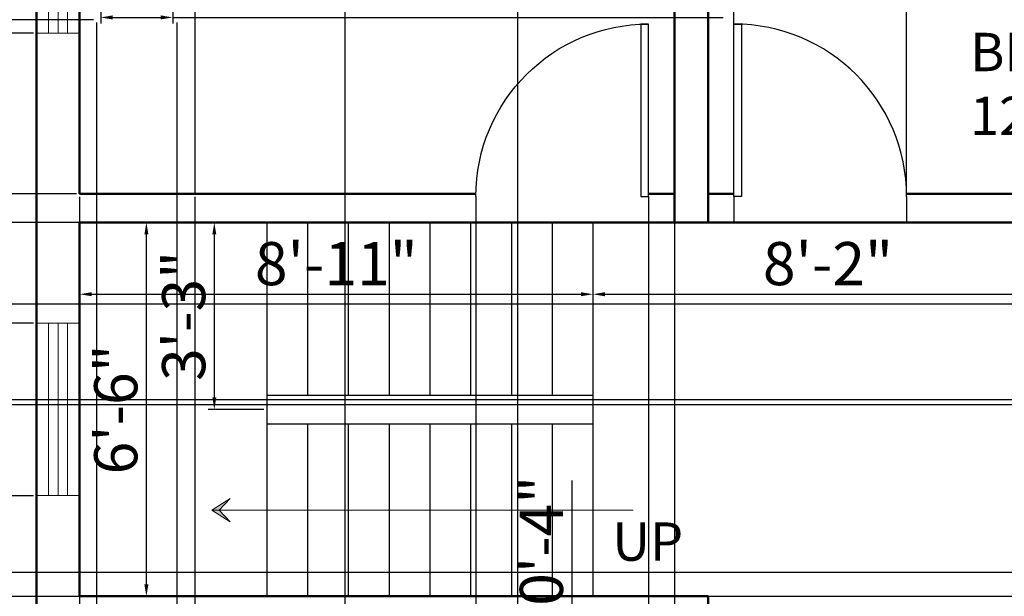
# Model space of a CAD drawing. Units: inches. Extents: x 2181 to 2717, y 1819 to 2296.
# Tile 3 of 5: x 2326 to 2531, y 2036 to 2157. Entities that reach past the tile are written whole.
import ezdxf

# ---------------------------------------------------------------- set-up
doc = ezdxf.new("R2010")
doc.units = ezdxf.units.IN
for name, color, linetype, lineweight in [('A-ANNO-DIMS', 2, 'Continuous', 13), ('A-ANNO-SYMB', 7, 'Continuous', 18), ('A-ANNO-SYMB-PATT', 7, 'Continuous', 18), ('A-ANNO-TEXT', 7, 'Continuous', 18), ('A-AREA-IDEN', 7, 'Continuous', 25), ('A-DOOR', 3, 'Continuous', 25), ('A-FLOR-CASE', 32, 'Continuous', 25), ('A-FLOR-STRS', 7, 'Continuous', 25), ('A-GLAZ', 4, 'Continuous', 18), ('A-WALL', 7, 'Continuous', 50)]:
    doc.layers.add(name, color=color, linetype=linetype, lineweight=lineweight)
doc.styles.get("Standard").update_dxf_attribs({"font": 'arial.ttf'})
doc.dimstyles.new('ISO-25', dxfattribs={"dimtxt": 9, "dimasz": 2.5, "dimexe": 1.25, "dimexo": 0.625, "dimtad": 1, "dimlunit": 3, "dimtxsty": 'Standard', "dimcen": 2.5, "dimadec": 0, "dimazin": 0, "dimtfac": 1, "dimtmove": 0, "dimatfit": 3, "dimfxl": 1, "dimarcsym": 0})

# ---------------------------------------------------------------- blocks, each defined once
blk = doc.blocks.new('*U2')
for p, q in [((0, 0), (0, -6)), ((40, 0), (40, -6))]:
    blk.add_line(p, q)
blk.add_lwpolyline([(0, 0), (0, 40), (1.75, 40), (1.75, 0)], close=True)
blk.add_arc((0, 0), 40, 0, 90)
blk = doc.blocks.new('*D10')
at = {"layer": 'A-ANNO-DIMS', "color": 0, "lineweight": -2, "transparency": 16777216}
for p, q in [((2338.97, 2114.2), (2353.51, 2114.2)), ((2352.26, 2038.7), (2352.26, 2111.7)), ((2338.97, 2036.2), (2353.51, 2036.2))]:
    blk.add_line(p, q, dxfattribs=at)
at = {"layer": 'A-ANNO-DIMS', "color": 0, "transparency": 16777216}
for points in [[(2351.84, 2111.7), (2352.68, 2111.7), (2352.26, 2114.2)], [(2351.84, 2038.7), (2352.68, 2038.7), (2352.26, 2036.2)]]:
    blk.add_solid(points, dxfattribs=at)
at = {"layer": 'Defpoints', "color": 0, "transparency": 16777216}
for p in [(2338.35, 2114.2), (2352.26, 2114.2), (2338.35, 2036.2)]:
    blk.add_point(p, dxfattribs=at)
at = {"layer": 'A-ANNO-DIMS', "color": 0, "transparency": 16777216, "insert": (2347.04, 2075.2), "char_height": 9, "attachment_point": 5, "rotation": 90}
blk.add_mtext('6\'-6"', dxfattribs=at)
blk = doc.blocks.new('*D11')
at = {"layer": 'A-ANNO-DIMS', "color": 0, "lineweight": -2, "transparency": 16777216}
for p, q in [((2376.72, 2114.2), (2365.17, 2114.2)), ((2366.42, 2111.7), (2366.42, 2077.7)), ((2376.72, 2075.2), (2365.17, 2075.2))]:
    blk.add_line(p, q, dxfattribs=at)
at = {"layer": 'A-ANNO-DIMS', "color": 0, "transparency": 16777216}
for points in [[(2366.01, 2111.7), (2366.84, 2111.7), (2366.42, 2114.2)], [(2366.01, 2077.7), (2366.84, 2077.7), (2366.42, 2075.2)]]:
    blk.add_solid(points, dxfattribs=at)
at = {"layer": 'Defpoints', "color": 0, "transparency": 16777216}
for p in [(2377.35, 2114.2), (2366.42, 2075.2), (2377.35, 2075.2)]:
    blk.add_point(p, dxfattribs=at)
at = {"layer": 'A-ANNO-DIMS', "color": 0, "transparency": 16777216, "insert": (2361.2, 2094.7), "char_height": 9, "attachment_point": 5, "rotation": 90}
blk.add_mtext('3\'-3"', dxfattribs=at)
blk = doc.blocks.new('*D12')
at = {"layer": 'A-ANNO-DIMS', "color": 0, "lineweight": -2, "transparency": 16777216}
for p, q in [((2338.35, 2113.58), (2338.35, 2097.98)), ((2445.35, 2113.58), (2445.35, 2097.98)), ((2340.85, 2099.23), (2442.85, 2099.23))]:
    blk.add_line(p, q, dxfattribs=at)
at = {"layer": 'A-ANNO-DIMS', "color": 0, "transparency": 16777216}
for points in [[(2340.85, 2099.65), (2340.85, 2098.81), (2338.35, 2099.23)], [(2442.85, 2099.65), (2442.85, 2098.81), (2445.35, 2099.23)]]:
    blk.add_solid(points, dxfattribs=at)
at = {"layer": 'Defpoints', "color": 0, "transparency": 16777216}
for p in [(2338.35, 2114.2), (2445.35, 2114.2), (2445.35, 2099.23)]:
    blk.add_point(p, dxfattribs=at)
at = {"layer": 'A-ANNO-DIMS', "color": 0, "transparency": 16777216, "insert": (2391.85, 2104.45), "char_height": 9, "attachment_point": 5}
blk.add_mtext('8\'-11"', dxfattribs=at)
blk = doc.blocks.new('*D13')
at = {"layer": 'A-ANNO-DIMS', "color": 0, "lineweight": -2, "transparency": 16777216}
for p, q in [((2445.35, 2113.58), (2445.35, 2097.98)), ((2543.35, 2113.58), (2543.35, 2097.98)), ((2447.85, 2099.23), (2540.85, 2099.23))]:
    blk.add_line(p, q, dxfattribs=at)
at = {"layer": 'A-ANNO-DIMS', "color": 0, "transparency": 16777216}
for points in [[(2447.85, 2099.65), (2447.85, 2098.81), (2445.35, 2099.23)], [(2540.85, 2099.65), (2540.85, 2098.81), (2543.35, 2099.23)]]:
    blk.add_solid(points, dxfattribs=at)
at = {"layer": 'Defpoints', "color": 0, "transparency": 16777216}
for p in [(2445.35, 2114.2), (2543.35, 2114.2), (2543.35, 2099.23)]:
    blk.add_point(p, dxfattribs=at)
at = {"layer": 'A-ANNO-DIMS', "color": 0, "transparency": 16777216, "insert": (2494.35, 2104.45), "char_height": 9, "attachment_point": 5}
blk.add_mtext('8\'-2"', dxfattribs=at)
blk = doc.blocks.new('WIN-60IN')
for p, q in [((0, 0), (0, 9)), ((60, 0), (60, 9)), ((60, 6.5), (0, 6.5)), ((60, 4.5), (0, 4.5)), ((60, 2.5), (0, 2.5))]:
    blk.add_line(p, q)
blk = doc.blocks.new('*D19')
at = {"layer": 'A-ANNO-DIMS', "color": 0, "lineweight": -2, "transparency": 16777216}
for p, q in [((2338.35, 1997.93), (2181.23, 1997.93)), ((2338.35, 1986.33), (2338.35, 1999.18)), ((2417.32, 1997.93), (2340.85, 1997.93)), ((2419.82, 1986.33), (2419.82, 1999.18))]:
    blk.add_line(p, q, dxfattribs=at)
at = {"layer": 'A-ANNO-DIMS', "color": 0, "transparency": 16777216}
for points in [[(2340.85, 1998.34), (2340.85, 1997.51), (2338.35, 1997.93)], [(2417.32, 1998.34), (2417.32, 1997.51), (2419.82, 1997.93)]]:
    blk.add_solid(points, dxfattribs=at)
at = {"layer": 'Defpoints', "color": 0, "transparency": 16777216}
for p in [(2338.35, 1997.93), (2338.35, 1985.7), (2419.82, 1985.7)]:
    blk.add_point(p, dxfattribs=at)
at = {"layer": 'A-ANNO-DIMS', "color": 0, "transparency": 16777216, "insert": (2258.54, 2003.48), "char_height": 9, "attachment_point": 5}
blk.add_mtext('QUEEN BED 6\'-9 1/2" TYP.', dxfattribs=at)
blk = doc.blocks.new('*D21')
at = {"layer": 'A-ANNO-DIMS', "color": 0, "lineweight": -2, "transparency": 16777216}
for p, q in [((2342.73, 2158.61), (2342.73, 2155.73)), ((2357.74, 2158.61), (2357.74, 2155.73)), ((2345.23, 2156.98), (2355.24, 2156.98)), ((2357.74, 2156.98), (2472.54, 2156.98))]:
    blk.add_line(p, q, dxfattribs=at)
at = {"layer": 'A-ANNO-DIMS', "color": 0, "transparency": 16777216}
for points in [[(2345.23, 2157.4), (2345.23, 2156.56), (2342.73, 2156.98)], [(2355.24, 2157.4), (2355.24, 2156.56), (2357.74, 2156.98)]]:
    blk.add_solid(points, dxfattribs=at)
at = {"layer": 'Defpoints', "color": 0, "transparency": 16777216}
for p in [(2342.73, 2159.23), (2357.74, 2159.23), (2357.74, 2156.98)]:
    blk.add_point(p, dxfattribs=at)
at = {"layer": 'A-ANNO-DIMS', "color": 0, "transparency": 16777216, "insert": (2416.39, 2162.2), "char_height": 9, "attachment_point": 5}
blk.add_mtext('BURNER 1\'-3" TYP.', dxfattribs=at)
blk = doc.blocks.new('*D27')
at = {"layer": 'A-ANNO-DIMS', "color": 0, "lineweight": -2, "transparency": 16777216}
for p, q in [((2328.72, 2093.2), (2306.75, 2093.2)), ((2308, 2090.7), (2308, 2059.7)), ((2328.72, 2057.2), (2306.75, 2057.2))]:
    blk.add_line(p, q, dxfattribs=at)
at = {"layer": 'A-ANNO-DIMS', "color": 0, "transparency": 16777216}
for points in [[(2307.58, 2090.7), (2308.41, 2090.7), (2308, 2093.2)], [(2307.58, 2059.7), (2308.41, 2059.7), (2308, 2057.2)]]:
    blk.add_solid(points, dxfattribs=at)
at = {"layer": 'Defpoints', "color": 0, "transparency": 16777216}
for p in [(2329.35, 2093.2), (2308, 2057.2), (2329.35, 2057.2)]:
    blk.add_point(p, dxfattribs=at)
at = {"layer": 'A-ANNO-DIMS', "color": 0, "transparency": 16777216, "insert": (2302.77, 2075.2), "char_height": 9, "attachment_point": 5, "rotation": 90}
blk.add_mtext('3\'-0"', dxfattribs=at)
blk = doc.blocks.new('*D28')
at = {"layer": 'A-ANNO-DIMS', "color": 0, "lineweight": -2, "transparency": 16777216}
for p, q in [((2328.72, 2153.7), (2306.75, 2153.7)), ((2308, 2095.7), (2308, 2151.2)), ((2328.72, 2093.2), (2306.75, 2093.2))]:
    blk.add_line(p, q, dxfattribs=at)
at = {"layer": 'A-ANNO-DIMS', "color": 0, "transparency": 16777216}
for points in [[(2307.58, 2151.2), (2308.41, 2151.2), (2308, 2153.7)], [(2307.58, 2095.7), (2308.41, 2095.7), (2308, 2093.2)]]:
    blk.add_solid(points, dxfattribs=at)
at = {"layer": 'Defpoints', "color": 0, "transparency": 16777216}
for p in [(2308, 2153.7), (2329.35, 2153.7), (2329.35, 2093.2)]:
    blk.add_point(p, dxfattribs=at)
at = {"layer": 'A-ANNO-DIMS', "color": 0, "transparency": 16777216, "insert": (2302.72, 2123.45), "char_height": 9, "attachment_point": 5, "rotation": 90}
blk.add_mtext('5\'-0 1/2"', dxfattribs=at)
blk = doc.blocks.new('*D40')
at = {"layer": 'A-ANNO-DIMS', "color": 0, "lineweight": -2, "transparency": 16777216}
for p, q in [((2474.75, 2120.83), (2474.75, 2278.8)), ((2510.75, 2120.83), (2510.75, 2278.8)), ((2477.25, 2277.55), (2508.25, 2277.55))]:
    blk.add_line(p, q, dxfattribs=at)
at = {"layer": 'A-ANNO-DIMS', "color": 0, "transparency": 16777216}
for points in [[(2477.25, 2277.97), (2477.25, 2277.14), (2474.75, 2277.55)], [(2508.25, 2277.97), (2508.25, 2277.14), (2510.75, 2277.55)]]:
    blk.add_solid(points, dxfattribs=at)
at = {"layer": 'Defpoints', "color": 0, "transparency": 16777216}
for p in [(2510.75, 2277.55), (2474.75, 2120.2), (2510.75, 2120.2)]:
    blk.add_point(p, dxfattribs=at)
at = {"layer": 'A-ANNO-DIMS', "color": 0, "transparency": 16777216, "insert": (2492.75, 2282.78), "char_height": 9, "attachment_point": 5}
blk.add_mtext('3\'-0"', dxfattribs=at)
blk = doc.blocks.new('*D41')
at = {"layer": 'A-ANNO-DIMS', "color": 0, "lineweight": -2, "transparency": 16777216}
for p, q in [((2338.35, 2119.58), (2338.35, 1825.6)), ((2362.35, 2119.58), (2362.35, 1825.6)), ((2340.85, 1826.85), (2359.85, 1826.85)), ((2362.35, 1826.85), (2390.17, 1826.85))]:
    blk.add_line(p, q, dxfattribs=at)
at = {"layer": 'A-ANNO-DIMS', "color": 0, "transparency": 16777216}
for points in [[(2340.85, 1827.27), (2340.85, 1826.44), (2338.35, 1826.85)], [(2359.85, 1827.27), (2359.85, 1826.44), (2362.35, 1826.85)]]:
    blk.add_solid(points, dxfattribs=at)
at = {"layer": 'Defpoints', "color": 0, "transparency": 16777216}
for p in [(2338.35, 2120.2), (2362.35, 2120.2), (2362.35, 1826.85)]:
    blk.add_point(p, dxfattribs=at)
at = {"layer": 'A-ANNO-DIMS', "color": 0, "transparency": 16777216, "insert": (2377.51, 1832.07), "char_height": 9, "attachment_point": 5}
blk.add_mtext('2\'-0"', dxfattribs=at)
blk = doc.blocks.new('*D43')
at = {"layer": 'A-ANNO-DIMS', "color": 0, "lineweight": -2, "transparency": 16777216}
for p, q in [((2393.61, 2225.64), (2393.61, 1825.6)), ((2429.61, 2225.64), (2429.61, 1825.6)), ((2396.11, 1826.85), (2427.11, 1826.85))]:
    blk.add_line(p, q, dxfattribs=at)
at = {"layer": 'A-ANNO-DIMS', "color": 0, "transparency": 16777216}
for points in [[(2396.11, 1827.27), (2396.11, 1826.44), (2393.61, 1826.85)], [(2427.11, 1827.27), (2427.11, 1826.44), (2429.61, 1826.85)]]:
    blk.add_solid(points, dxfattribs=at)
at = {"layer": 'Defpoints', "color": 0, "transparency": 16777216}
for p in [(2393.61, 2226.26), (2429.61, 2226.26), (2429.61, 1826.85)]:
    blk.add_point(p, dxfattribs=at)
at = {"layer": 'A-ANNO-DIMS', "color": 0, "transparency": 16777216, "insert": (2411.61, 1832.08), "char_height": 9, "attachment_point": 5}
blk.add_mtext('3\'-0"', dxfattribs=at)
blk = doc.blocks.new('*D45')
at = {"layer": 'A-ANNO-DIMS', "color": 0, "lineweight": -2, "transparency": 16777216}
for p, q in [((2429.61, 2225.64), (2429.61, 1825.6)), ((2462.35, 2222.58), (2462.35, 1825.6)), ((2432.11, 1826.85), (2459.85, 1826.85)), ((2462.35, 1826.85), (2511.15, 1826.85))]:
    blk.add_line(p, q, dxfattribs=at)
at = {"layer": 'A-ANNO-DIMS', "color": 0, "transparency": 16777216}
for points in [[(2432.11, 1827.27), (2432.11, 1826.44), (2429.61, 1826.85)], [(2459.85, 1827.27), (2459.85, 1826.44), (2462.35, 1826.85)]]:
    blk.add_solid(points, dxfattribs=at)
at = {"layer": 'Defpoints', "color": 0, "transparency": 16777216}
for p in [(2429.61, 2226.26), (2462.35, 2223.2), (2462.35, 1826.85)]:
    blk.add_point(p, dxfattribs=at)
at = {"layer": 'A-ANNO-DIMS', "color": 0, "transparency": 16777216, "insert": (2488, 1832.13), "char_height": 9, "attachment_point": 5}
blk.add_mtext('2\'-8 1/2"', dxfattribs=at)
blk = doc.blocks.new('*D46')
at = {"layer": 'A-ANNO-DIMS', "color": 0, "lineweight": -2, "transparency": 16777216}
for p, q in [((2341.24, 2198.7), (2306.75, 2198.7)), ((2308, 2159.01), (2308, 2196.2)), ((2341.24, 2156.51), (2306.75, 2156.51))]:
    blk.add_line(p, q, dxfattribs=at)
at = {"layer": 'A-ANNO-DIMS', "color": 0, "transparency": 16777216}
for points in [[(2307.58, 2196.2), (2308.41, 2196.2), (2308, 2198.7)], [(2307.58, 2159.01), (2308.41, 2159.01), (2308, 2156.51)]]:
    blk.add_solid(points, dxfattribs=at)
at = {"layer": 'Defpoints', "color": 0, "transparency": 16777216}
for p in [(2308, 2198.7), (2341.86, 2198.7), (2341.86, 2156.51)]:
    blk.add_point(p, dxfattribs=at)
at = {"layer": 'A-ANNO-DIMS', "color": 0, "transparency": 16777216, "insert": (2302.77, 2177.61), "char_height": 9, "attachment_point": 5, "rotation": 90}
blk.add_mtext('3\'-6"', dxfattribs=at)
blk = doc.blocks.new('*D47')
at = {"layer": 'A-ANNO-DIMS', "color": 0, "lineweight": -2, "transparency": 16777216}
for p, q in [((2341.86, 2155.89), (2341.86, 1825.6)), ((2358.61, 2155.89), (2358.61, 1825.6)), ((2344.36, 1826.85), (2356.11, 1826.85)), ((2358.61, 1826.85), (2406.41, 1826.85))]:
    blk.add_line(p, q, dxfattribs=at)
at = {"layer": 'A-ANNO-DIMS', "color": 0, "transparency": 16777216}
for points in [[(2344.36, 1827.27), (2344.36, 1826.44), (2341.86, 1826.85)], [(2356.11, 1827.27), (2356.11, 1826.44), (2358.61, 1826.85)]]:
    blk.add_solid(points, dxfattribs=at)
at = {"layer": 'Defpoints', "color": 0, "transparency": 16777216}
for p in [(2341.86, 2156.51), (2358.61, 2156.51), (2358.61, 1826.85)]:
    blk.add_point(p, dxfattribs=at)
at = {"layer": 'A-ANNO-DIMS', "color": 0, "transparency": 16777216, "insert": (2383.76, 1832.13), "char_height": 9, "attachment_point": 5}
blk.add_mtext('1\'-4 1/2"', dxfattribs=at)
blk = doc.blocks.new('*D48')
at = {"layer": 'A-ANNO-DIMS', "color": 0, "lineweight": -2, "transparency": 16777216}
for p, q in [((2308, 2156.51), (2308, 2205.15)), ((2341.24, 2156.51), (2306.75, 2156.51)), ((2308, 2122.7), (2308, 2154.01)), ((2337.72, 2120.2), (2306.75, 2120.2))]:
    blk.add_line(p, q, dxfattribs=at)
at = {"layer": 'A-ANNO-DIMS', "color": 0, "transparency": 16777216}
for points in [[(2307.58, 2154.01), (2308.41, 2154.01), (2308, 2156.51)], [(2307.58, 2122.7), (2308.41, 2122.7), (2308, 2120.2)]]:
    blk.add_solid(points, dxfattribs=at)
at = {"layer": 'Defpoints', "color": 0, "transparency": 16777216}
for p in [(2308, 2156.51), (2341.86, 2156.51), (2338.35, 2120.2)]:
    blk.add_point(p, dxfattribs=at)
at = {"layer": 'A-ANNO-DIMS', "color": 0, "transparency": 16777216, "insert": (2302.71, 2182.08), "char_height": 9, "attachment_point": 5, "rotation": 90}
blk.add_mtext('3\'-0 1/2"', dxfattribs=at)
blk = doc.blocks.new('*D50')
at = {"layer": 'A-ANNO-DIMS', "color": 0, "lineweight": -2, "transparency": 16777216}
for p, q in [((2308, 2097.13), (2308, 2123.96)), ((2611.72, 2097.13), (2306.75, 2097.13)), ((2308, 2078.63), (2308, 2094.63)), ((2611.72, 2076.13), (2306.75, 2076.13))]:
    blk.add_line(p, q, dxfattribs=at)
at = {"layer": 'A-ANNO-DIMS', "color": 0, "transparency": 16777216}
for points in [[(2307.58, 2094.63), (2308.41, 2094.63), (2308, 2097.13)], [(2307.58, 2078.63), (2308.41, 2078.63), (2308, 2076.13)]]:
    blk.add_solid(points, dxfattribs=at)
at = {"layer": 'Defpoints', "color": 0, "transparency": 16777216}
for p in [(2308, 2097.13), (2612.35, 2097.13), (2612.35, 2076.13)]:
    blk.add_point(p, dxfattribs=at)
at = {"layer": 'A-ANNO-DIMS', "color": 0, "transparency": 16777216, "insert": (2302.78, 2111.79), "char_height": 9, "attachment_point": 5, "rotation": 90}
blk.add_mtext('1\'-9"', dxfattribs=at)
blk = doc.blocks.new('*D52')
at = {"layer": 'A-ANNO-DIMS', "color": 0, "lineweight": -2, "transparency": 16777216}
for p, q in [((2542.72, 2077.19), (2306.75, 2077.19)), ((2308, 2043.69), (2308, 2074.69)), ((2542.72, 2041.19), (2306.75, 2041.19))]:
    blk.add_line(p, q, dxfattribs=at)
at = {"layer": 'A-ANNO-DIMS', "color": 0, "transparency": 16777216}
for points in [[(2307.58, 2074.69), (2308.41, 2074.69), (2308, 2077.19)], [(2307.58, 2043.69), (2308.41, 2043.69), (2308, 2041.19)]]:
    blk.add_solid(points, dxfattribs=at)
at = {"layer": 'Defpoints', "color": 0, "transparency": 16777216}
for p in [(2308, 2077.19), (2543.35, 2077.19), (2543.35, 2041.19)]:
    blk.add_point(p, dxfattribs=at)
at = {"layer": 'A-ANNO-DIMS', "color": 0, "transparency": 16777216, "insert": (2302.77, 2059.19), "char_height": 9, "attachment_point": 5, "rotation": 90}
blk.add_mtext('3\'-0"', dxfattribs=at)
blk = doc.blocks.new('*D53')
at = {"layer": 'A-ANNO-DIMS', "color": 0, "lineweight": -2, "transparency": 16777216}
for p, q in [((2308, 2043.69), (2308, 2046.19)), ((2549.72, 2041.19), (2306.75, 2041.19)), ((2308, 2041.19), (2308, 2036.2)), ((2549.72, 2036.2), (2306.75, 2036.2)), ((2308, 2033.7), (2308, 2006.03))]:
    blk.add_line(p, q, dxfattribs=at)
at = {"layer": 'A-ANNO-DIMS', "color": 0, "transparency": 16777216}
for points in [[(2307.58, 2043.69), (2308.41, 2043.69), (2308, 2041.19)], [(2307.58, 2033.7), (2308.41, 2033.7), (2308, 2036.2)]]:
    blk.add_solid(points, dxfattribs=at)
at = {"layer": 'Defpoints', "color": 0, "transparency": 16777216}
for p in [(2550.35, 2041.19), (2308, 2036.2), (2550.35, 2036.2)]:
    blk.add_point(p, dxfattribs=at)
at = {"layer": 'A-ANNO-DIMS', "color": 0, "transparency": 16777216, "insert": (2302.78, 2018.62), "char_height": 9, "attachment_point": 5, "rotation": 90}
blk.add_mtext('0\'-5"', dxfattribs=at)
blk = doc.blocks.new('*D56')
at = {"layer": 'A-ANNO-DIMS', "color": 0, "lineweight": -2, "transparency": 16777216}
for p, q in [((2549.72, 2114.2), (2306.75, 2114.2)), ((2308, 2038.7), (2308, 2111.7)), ((2549.72, 2036.2), (2306.75, 2036.2))]:
    blk.add_line(p, q, dxfattribs=at)
at = {"layer": 'A-ANNO-DIMS', "color": 0, "transparency": 16777216}
for points in [[(2307.58, 2111.7), (2308.41, 2111.7), (2308, 2114.2)], [(2307.58, 2038.7), (2308.41, 2038.7), (2308, 2036.2)]]:
    blk.add_solid(points, dxfattribs=at)
at = {"layer": 'Defpoints', "color": 0, "transparency": 16777216}
for p in [(2308, 2114.2), (2550.35, 2114.2), (2550.35, 2036.2)]:
    blk.add_point(p, dxfattribs=at)
at = {"layer": 'A-ANNO-DIMS', "color": 0, "transparency": 16777216, "insert": (2302.78, 2075.2), "char_height": 9, "attachment_point": 5, "rotation": 90}
blk.add_mtext('6\'-6"', dxfattribs=at)
blk = doc.blocks.new('*D57')
at = {"layer": 'A-ANNO-DIMS', "color": 0, "lineweight": -2, "transparency": 16777216}
for p, q in [((2456.94, 2119.58), (2456.94, 1825.6)), ((2462.35, 2119.58), (2462.35, 1825.6)), ((2454.44, 1826.85), (2405.8, 1826.85)), ((2462.35, 1826.85), (2456.94, 1826.85)), ((2464.85, 1826.85), (2467.35, 1826.85))]:
    blk.add_line(p, q, dxfattribs=at)
at = {"layer": 'A-ANNO-DIMS', "color": 0, "transparency": 16777216}
for points in [[(2454.44, 1827.27), (2454.44, 1826.44), (2456.94, 1826.85)], [(2464.85, 1827.27), (2464.85, 1826.44), (2462.35, 1826.85)]]:
    blk.add_solid(points, dxfattribs=at)
at = {"layer": 'Defpoints', "color": 0, "transparency": 16777216}
for p in [(2456.94, 2120.2), (2462.35, 2120.2), (2456.94, 1826.85)]:
    blk.add_point(p, dxfattribs=at)
at = {"layer": 'A-ANNO-DIMS', "color": 0, "transparency": 16777216, "insert": (2428.87, 1832.13), "char_height": 9, "attachment_point": 5}
blk.add_mtext('0\'-5 1/2"', dxfattribs=at)
blk = doc.blocks.new('*D58')
at = {"layer": 'A-ANNO-DIMS', "color": 0, "lineweight": -2, "transparency": 16777216}
for p, q in [((2420.94, 2119.58), (2420.94, 1825.6)), ((2456.94, 2119.58), (2456.94, 1825.6)), ((2423.44, 1826.85), (2454.44, 1826.85))]:
    blk.add_line(p, q, dxfattribs=at)
at = {"layer": 'A-ANNO-DIMS', "color": 0, "transparency": 16777216}
for points in [[(2423.44, 1827.27), (2423.44, 1826.44), (2420.94, 1826.85)], [(2454.44, 1827.27), (2454.44, 1826.44), (2456.94, 1826.85)]]:
    blk.add_solid(points, dxfattribs=at)
at = {"layer": 'Defpoints', "color": 0, "transparency": 16777216}
for p in [(2420.94, 2120.2), (2456.94, 2120.2), (2456.94, 1826.85)]:
    blk.add_point(p, dxfattribs=at)
at = {"layer": 'A-ANNO-DIMS', "color": 0, "transparency": 16777216, "insert": (2438.94, 1832.08), "char_height": 9, "attachment_point": 5}
blk.add_mtext('3\'-0"', dxfattribs=at)
blk = doc.blocks.new('*D60')
at = {"layer": 'A-ANNO-DIMS', "color": 0, "lineweight": -2, "transparency": 16777216}
for p, q in [((2441, 2032.7), (2441, 2060.38)), ((2461.72, 2030.2), (2439.75, 2030.2)), ((2441, 2026.24), (2441, 2030.2)), ((2461.72, 2026.24), (2439.75, 2026.24)), ((2441, 2023.74), (2441, 2021.24))]:
    blk.add_line(p, q, dxfattribs=at)
at = {"layer": 'A-ANNO-DIMS', "color": 0, "transparency": 16777216}
for points in [[(2440.58, 2032.7), (2441.41, 2032.7), (2441, 2030.2)], [(2440.58, 2023.74), (2441.41, 2023.74), (2441, 2026.24)]]:
    blk.add_solid(points, dxfattribs=at)
at = {"layer": 'Defpoints', "color": 0, "transparency": 16777216}
for p in [(2441, 2030.2), (2462.35, 2030.2), (2462.35, 2026.24)]:
    blk.add_point(p, dxfattribs=at)
at = {"layer": 'A-ANNO-DIMS', "color": 0, "transparency": 16777216, "insert": (2435.78, 2047.79), "char_height": 9, "attachment_point": 5, "rotation": 90}
blk.add_mtext('0\'-4"', dxfattribs=at)
blk = doc.blocks.new('*D61')
at = {"layer": 'A-ANNO-DIMS', "color": 0, "lineweight": -2, "transparency": 16777216}
for p, q in [((2469.35, 2120.83), (2469.35, 2278.8)), ((2474.75, 2120.83), (2474.75, 2278.8)), ((2466.85, 2277.55), (2464.35, 2277.55)), ((2469.35, 2277.55), (2474.75, 2277.55)), ((2477.25, 2277.55), (2525.9, 2277.55))]:
    blk.add_line(p, q, dxfattribs=at)
at = {"layer": 'A-ANNO-DIMS', "color": 0, "transparency": 16777216}
for points in [[(2466.85, 2277.97), (2466.85, 2277.14), (2469.35, 2277.55)], [(2477.25, 2277.97), (2477.25, 2277.14), (2474.75, 2277.55)]]:
    blk.add_solid(points, dxfattribs=at)
at = {"layer": 'Defpoints', "color": 0, "transparency": 16777216}
for p in [(2474.75, 2277.55), (2469.35, 2120.2), (2474.75, 2120.2)]:
    blk.add_point(p, dxfattribs=at)
at = {"layer": 'A-ANNO-DIMS', "color": 0, "transparency": 16777216, "insert": (2502.82, 2282.83), "char_height": 9, "attachment_point": 5}
blk.add_mtext('0\'-5 1/2"', dxfattribs=at)

msp = doc.modelspace()

# ---------------------------------------------------------------- hatches: boundary and pattern name
at = {"layer": 'A-ANNO-SYMB-PATT'}
h = msp.add_hatch(color=256, dxfattribs=at)
h.dxf.hatch_style = 1
h.paths.add_polyline_path([(2369.701, 2056.636), (2365.876, 2054.205), (2367.443, 2054.205)])
h.paths.add_polyline_path([(2367.443, 2054.205), (2365.876, 2054.205), (2369.701, 2051.774)])

# ---------------------------------------------------------------- linework, layer by layer
at = {"layer": 'A-ANNO-SYMB'}
for p, q in [((2365.876, 2054.205), (2369.701, 2056.636)), ((2369.701, 2056.636), (2367.443, 2054.205)), ((2453.746, 2054.205), (2365.876, 2054.205)), ((2365.876, 2054.205), (2369.701, 2051.774)), ((2369.701, 2051.774), (2367.443, 2054.205))]:
    msp.add_line(p, q, dxfattribs=at)
at = {"layer": 'A-DOOR'}
msp.add_line((2474.75, 2115.486), (2474.842, 2115.486), dxfattribs=at)
at = {"layer": 'A-FLOR-CASE'}
msp.add_line((2362.346, 2223.205), (2362.346, 2120.205), dxfattribs=at)
at = {"layer": 'A-FLOR-STRS'}
for p, q in [((2377.346, 2114.205), (2377.346, 2036.205)), ((2385.846, 2114.205), (2385.846, 2078.205)), ((2394.346, 2114.205), (2394.346, 2078.205)), ((2402.846, 2114.205), (2402.846, 2078.205)), ((2411.346, 2114.205), (2411.346, 2078.205)), ((2419.846, 2114.205), (2419.846, 2078.205)), ((2428.346, 2114.205), (2428.346, 2078.205)), ((2436.846, 2114.205), (2436.846, 2078.205)), ((2445.346, 2114.205), (2445.346, 2036.205)), ((2377.346, 2078.205), (2445.346, 2078.205)), ((2377.346, 2072.205), (2445.346, 2072.205)), ((2385.846, 2072.205), (2385.846, 2036.205)), ((2394.346, 2072.205), (2394.346, 2036.205)), ((2402.846, 2072.205), (2402.846, 2036.205)), ((2411.346, 2072.205), (2411.346, 2036.205)), ((2419.846, 2072.205), (2419.846, 2036.205)), ((2428.346, 2072.205), (2428.346, 2036.205)), ((2436.846, 2072.205), (2436.846, 2036.205))]:
    msp.add_line(p, q, dxfattribs=at)
at = {"layer": 'A-GLAZ'}
for p, q in [((2338.346, 2093.205), (2329.346, 2093.205)), ((2331.846, 2093.205), (2331.846, 2057.205)), ((2333.846, 2093.205), (2333.846, 2057.205)), ((2335.846, 2093.205), (2335.846, 2057.205)), ((2338.346, 2057.205), (2329.346, 2057.205))]:
    msp.add_line(p, q, dxfattribs=at)
at = {"layer": 'A-WALL'}
for p, q in [((2329.346, 2256.205), (2329.346, 1872.205)), ((2338.346, 2247.205), (2338.346, 2120.205)), ((2462.346, 2247.205), (2462.346, 2120.205)), ((2469.346, 2247.205), (2469.346, 2120.205)), ((2338.346, 2120.205), (2420.942, 2120.205)), ((2456.942, 2120.205), (2462.346, 2120.205)), ((2462.346, 2120.205), (2462.346, 2114.205)), ((2469.346, 2120.205), (2474.75, 2120.205)), ((2469.346, 2114.205), (2469.346, 2120.205)), ((2510.745, 2120.205), (2620.346, 2120.205)), ((2338.346, 2114.205), (2620.346, 2114.205)), ((2338.346, 2114.205), (2338.346, 2036.205)), ((2338.346, 2036.205), (2469.346, 2036.205)), ((2469.346, 2036.205), (2469.346, 1881.205))]:
    msp.add_line(p, q, dxfattribs=at)

# ---------------------------------------------------------------- block references
at = {"layer": 'A-DOOR', "yscale": 0.9, "zscale": 0.9}
for p, xscale in [((2456.942, 2119.605), -0.9), ((2474.75, 2119.605), 0.9)]:
    msp.add_blockref('*U2', p, dxfattribs=dict(at, xscale=xscale))
at = {"layer": 'A-GLAZ', "rotation": 89.99999999999747}
msp.add_blockref('WIN-60IN', (2338.346, 2153.704), dxfattribs=at)

# ---------------------------------------------------------------- texts
at = {"layer": 'A-ANNO-TEXT', "insert": (2449.39, 2051.623), "char_height": 8, "attachment_point": 1}
msp.add_mtext_dynamic_manual_height_columns('UP', width=10.96422, gutter_width=12.5, heights=[0], dxfattribs=at)
at = {"layer": 'A-AREA-IDEN', "insert": (2523.994, 2153.766), "char_height": 8, "attachment_point": 1}
msp.add_mtext_dynamic_manual_height_columns('BEDROOM-1\\P12\'7"*10\'7"', width=37.99236, gutter_width=12.5, heights=[0], dxfattribs=at)

# ---------------------------------------------------------------- dimensions: what is measured, and where the dimension line sits
at = {"layer": 'A-ANNO-DIMS'}
for base, p1, p2, override, picture, middle in [((2474.75, 2277.555), (2469.346, 2120.205), (2474.75, 2120.205), {"dimdec": 1, "dimlfac": 1, "dimrnd": 0, "dimzin": 1, "dimdsep": 46, "dimlunit": 4, "dimfrac": 2}, '*D61', (2502.823, 2282.833)), ((2510.745, 2277.555), (2474.75, 2120.205), (2510.745, 2120.205), {"dimdec": 1, "dimlfac": 1, "dimrnd": 0, "dimzin": 1, "dimdsep": 46, "dimlunit": 4, "dimfrac": 2}, '*D40', (2492.748, 2282.778)), ((2429.61, 1826.855), (2393.61, 2226.263), (2429.61, 2226.263), {"dimdec": 1, "dimlfac": 1, "dimrnd": 0, "dimzin": 1, "dimdsep": 46, "dimlunit": 4, "dimfrac": 2}, '*D43', (2411.61, 1832.078)), ((2462.346, 1826.855), (2429.61, 2226.263), (2462.346, 2223.205), {"dimdec": 1, "dimlfac": 1, "dimrnd": 0, "dimzin": 1, "dimdsep": 46, "dimlunit": 4, "dimfrac": 2}, '*D45', (2487.996, 1832.133)), ((2358.609, 1826.855), (2341.861, 2156.51), (2358.609, 2156.51), {"dimdec": 1, "dimlfac": 1, "dimrnd": 0, "dimzin": 1, "dimdsep": 46, "dimlunit": 4, "dimfrac": 2}, '*D47', (2383.758, 1832.133)), ((2362.346, 1826.855), (2338.346, 2120.205), (2362.346, 2120.205), {"dimdec": 1, "dimlfac": 1, "dimrnd": 0, "dimzin": 1, "dimdsep": 46, "dimlunit": 4, "dimfrac": 2}, '*D41', (2377.51, 1832.075)), ((2456.942, 1826.855), (2462.346, 2120.205), (2456.942, 2120.205), {"dimdec": 1, "dimlfac": 1, "dimrnd": 0, "dimzin": 1, "dimdsep": 46, "dimlunit": 4, "dimfrac": 2}, '*D57', (2428.87, 1832.133)), ((2456.942, 1826.855), (2420.942, 2120.205), (2456.942, 2120.205), {"dimdec": 1, "dimlfac": 1, "dimrnd": 0, "dimzin": 1, "dimdsep": 46, "dimlunit": 4, "dimfrac": 2}, '*D58', (2438.942, 1832.078)), ((2445.346, 2099.229), (2338.346, 2114.205), (2445.346, 2114.205), {"dimclrd": 0, "dimclre": 0, "dimclrt": 0}, '*D12', (2391.846, 2104.449)), ((2543.346, 2099.229), (2445.346, 2114.205), (2543.346, 2114.205), {"dimclrd": 0, "dimclre": 0, "dimclrt": 0}, '*D13', (2494.346, 2104.449))]:
    dim = msp.add_linear_dim(base=base, p1=p1, p2=p2, dimstyle='ISO-25', override=override, dxfattribs=at)
    dim.commit()
    dim.dimension.update_dxf_attribs({"geometry": picture, "text_midpoint": middle})
for base, p1, p2, override, picture, middle in [((2307.996, 2156.51), (2338.346, 2120.205), (2341.861, 2156.51), {"dimdec": 1, "dimlfac": 1, "dimrnd": 0, "dimzin": 1, "dimdsep": 46, "dimlunit": 4, "dimfrac": 2}, '*D48', (2302.715, 2182.08)), ((2307.996, 2198.704), (2341.861, 2156.51), (2341.861, 2198.704), {"dimdec": 1, "dimlfac": 1, "dimrnd": 0, "dimzin": 1, "dimdsep": 46, "dimlunit": 4, "dimfrac": 2}, '*D46', (2302.773, 2177.607)), ((2307.996, 2153.705), (2329.346, 2093.205), (2329.346, 2153.705), {"dimdec": 1, "dimlfac": 1, "dimrnd": 0, "dimzin": 1, "dimdsep": 46, "dimlunit": 4, "dimfrac": 2}, '*D28', (2302.718, 2123.455)), ((2307.996, 2097.128), (2612.346, 2076.128), (2612.346, 2097.128), {"dimdec": 1, "dimlfac": 1, "dimrnd": 0, "dimzin": 1, "dimdsep": 46, "dimlunit": 4, "dimfrac": 2}, '*D50', (2302.776, 2111.792)), ((2307.996, 2114.205), (2550.346, 2036.205), (2550.346, 2114.205), {"dimdec": 1, "dimlfac": 1, "dimrnd": 0, "dimzin": 1, "dimdsep": 46, "dimlunit": 4, "dimfrac": 2}, '*D56', (2302.776, 2075.205)), ((2352.259, 2114.205), (2338.346, 2036.205), (2338.346, 2114.205), {"dimclrd": 0, "dimclre": 0, "dimclrt": 0}, '*D10', (2347.039, 2075.205)), ((2366.425, 2075.205), (2377.346, 2114.205), (2377.346, 2075.205), {"dimclrd": 0, "dimclre": 0, "dimclrt": 0}, '*D11', (2361.201, 2094.705)), ((2307.996, 2057.205), (2329.346, 2093.205), (2329.346, 2057.205), {"dimdec": 1, "dimlfac": 1, "dimrnd": 0, "dimzin": 1, "dimdsep": 46, "dimlunit": 4, "dimfrac": 2}, '*D27', (2302.773, 2075.205)), ((2307.996, 2077.187), (2543.346, 2041.187), (2543.346, 2077.187), {"dimdec": 1, "dimlfac": 1, "dimrnd": 0, "dimzin": 1, "dimdsep": 46, "dimlunit": 4, "dimfrac": 2}, '*D52', (2302.773, 2059.187)), ((2440.996, 2030.205), (2462.346, 2026.245), (2462.346, 2030.205), {"dimdec": 1, "dimlfac": 1, "dimrnd": 0, "dimzin": 1, "dimdsep": 46, "dimlunit": 4, "dimfrac": 2}, '*D60', (2435.776, 2047.792)), ((2307.996, 2036.205), (2550.346, 2041.187), (2550.346, 2036.205), {"dimdec": 1, "dimlfac": 1, "dimrnd": 0, "dimzin": 1, "dimdsep": 46, "dimlunit": 4, "dimfrac": 2}, '*D53', (2302.776, 2018.617))]:
    dim = msp.add_linear_dim(base=base, p1=p1, p2=p2, angle=90, dimstyle='ISO-25', override=override, dxfattribs=at)
    dim.commit()
    dim.dimension.update_dxf_attribs({"geometry": picture, "text_midpoint": middle})
dim = msp.add_linear_dim(base=(2357.741, 2156.979), p1=(2342.729, 2159.231), p2=(2357.741, 2159.231), text='BURNER <> TYP.', dimstyle='ISO-25', override={"dimdec": 1, "dimlfac": 1, "dimrnd": 0, "dimzin": 1, "dimdsep": 46, "dimlunit": 4, "dimfrac": 2}, dxfattribs=at)
dim.commit()
dim.dimension.update_dxf_attribs({"geometry": '*D21', "text_midpoint": (2416.388, 2162.203)})
dim = msp.add_linear_dim(base=(2338.346, 1997.926), p1=(2419.819, 1985.705), p2=(2338.346, 1985.705), angle=180, text='QUEEN BED <> TYP.', dimstyle='ISO-25', override={"dimdec": 1, "dimlfac": 1, "dimrnd": 0, "dimzin": 1, "dimdsep": 46, "dimlunit": 4, "dimfrac": 2}, dxfattribs=at)
dim.commit()
dim.dimension.update_dxf_attribs({"geometry": '*D19', "text_midpoint": (2258.54, 2003.48)})

doc.saveas('drawing.dxf')
